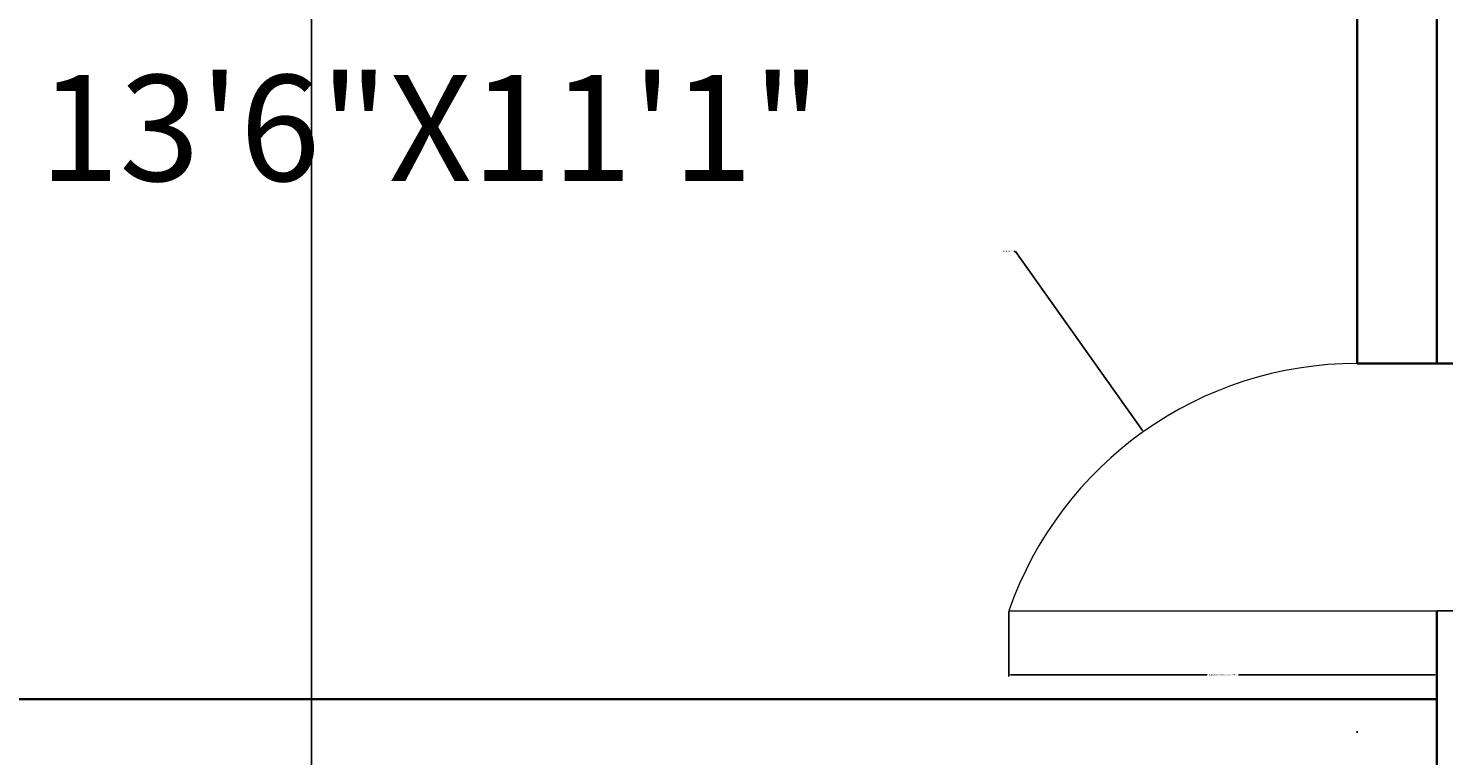
# Model space of a CAD drawing. Units: feet. Extents: x 5816 to 6644, y 25475 to 26788.
# Tile 12 of 23: x 5922 to 6082, y 26514 to 26597. Entities that reach past the tile are written whole.
import ezdxf

# ---------------------------------------------------------------- set-up
doc = ezdxf.new("R2010")
doc.units = ezdxf.units.FT
for name, color, linetype, lineweight in [('A-ANNO-DIMS', 2, 'Continuous', 13), ('A-DOOR', 3, 'Continuous', 18), ('A-WALL', 7, 'Continuous', 35)]:
    doc.layers.add(name, color=color, linetype=linetype, lineweight=lineweight)
doc.styles.get("Standard").update_dxf_attribs({"font": 'arial.ttf'})
doc.dimstyles.get("Standard").update_dxf_attribs({"dimtxt": 0.18, "dimasz": 0.18, "dimexe": 0.18, "dimexo": 0.0625, "dimgap": 0.09, "dimtad": 0, "dimtih": 1, "dimtoh": 1, "dimdec": 4, "dimzin": 0, "dimdsep": 46, "dimtxsty": 'Standard', "dimcen": 0.09, "dimadec": 0, "dimazin": 0, "dimtfac": 1, "dimtdec": 4, "dimtofl": 0, "dimtmove": 0, "dimatfit": 3, "dimfxl": 1, "dimtolj": 1, "dimtzin": 0, "dimarcsym": 0})

# ---------------------------------------------------------------- blocks, each defined once
blk = doc.blocks.new('DOOR-BEDROOM-BALCONY')
blk.add_line((-48.41, 0), (0, 0))
blk.add_arc((-9, -13.73), 41.74, 90, 160.7878)
blk = doc.blocks.new('*D23')
at = {"layer": 'A-ANNO-DIMS', "color": 0, "lineweight": -2, "transparency": 16777216}
for p, q in [((6032.9, 26530.52), (6032.9, 26523.14)), ((6081.31, 26530.52), (6081.31, 26523.14)), ((6033.08, 26523.32), (6055.32, 26523.32)), ((6081.13, 26523.32), (6058.89, 26523.32))]:
    blk.add_line(p, q, dxfattribs=at)
at = {"layer": 'A-ANNO-DIMS', "color": 0, "transparency": 16777216}
for points in [[(6033.08, 26523.35), (6033.08, 26523.29), (6032.9, 26523.32)], [(6081.13, 26523.35), (6081.13, 26523.29), (6081.31, 26523.32)]]:
    blk.add_solid(points, dxfattribs=at)
at = {"layer": 'Defpoints', "color": 0, "transparency": 16777216}
for p in [(6032.9, 26530.58), (6081.31, 26530.58), (6081.31, 26523.32)]:
    blk.add_point(p, dxfattribs=at)
at = {"layer": 'A-ANNO-DIMS', "color": 0, "transparency": 16777216, "insert": (6057.11, 26523.32), "char_height": 0.18, "attachment_point": 5}
blk.add_mtext('\\A1;BALCONY BR DOOR 48 TYP.', dxfattribs=at)
blk = doc.blocks.new('*D24')
at = {"layer": 'A-ANNO-DIMS', "color": 0, "lineweight": -2, "transparency": 16777216}
for p, q in [((6081.37, 26558.58), (6088.75, 26558.58)), ((6088.57, 26558.4), (6088.57, 26544.77)), ((6088.57, 26530.76), (6088.57, 26544.4)), ((6081.37, 26530.58), (6088.75, 26530.58))]:
    blk.add_line(p, q, dxfattribs=at)
at = {"layer": 'A-ANNO-DIMS', "color": 0, "transparency": 16777216}
for points in [[(6088.54, 26558.4), (6088.6, 26558.4), (6088.57, 26558.58)], [(6088.54, 26530.76), (6088.6, 26530.76), (6088.57, 26530.58)]]:
    blk.add_solid(points, dxfattribs=at)
at = {"layer": 'Defpoints', "color": 0, "transparency": 16777216}
for p in [(6081.31, 26558.58), (6088.57, 26558.58), (6081.31, 26530.58)]:
    blk.add_point(p, dxfattribs=at)
at = {"layer": 'A-ANNO-DIMS', "color": 0, "transparency": 16777216, "insert": (6088.57, 26544.58), "char_height": 0.18, "attachment_point": 5}
blk.add_mtext('\\A1;28 TYP.', dxfattribs=at)
blk = doc.blocks.new('*D58')
at = {"layer": 'A-ANNO-DIMS', "color": 0, "lineweight": -2, "transparency": 16777216}
for p, q in [((5953.98, 26168.65), (5953.98, 26787.91)), ((5954.16, 26787.73), (6030.2, 26787.73)), ((6106.8, 26787.73), (6030.76, 26787.73)), ((6106.98, 26168.71), (6106.98, 26787.91))]:
    blk.add_line(p, q, dxfattribs=at)
at = {"layer": 'A-ANNO-DIMS', "color": 0, "transparency": 16777216}
for points in [[(5954.16, 26787.76), (5954.16, 26787.7), (5953.98, 26787.73)], [(6106.8, 26787.76), (6106.8, 26787.7), (6106.98, 26787.73)]]:
    blk.add_solid(points, dxfattribs=at)
at = {"layer": 'Defpoints', "color": 0, "transparency": 16777216}
for p in [(6106.98, 26787.73), (5953.98, 26168.58), (6106.98, 26168.65)]:
    blk.add_point(p, dxfattribs=at)
at = {"layer": 'A-ANNO-DIMS', "color": 0, "transparency": 16777216, "insert": (6030.48, 26787.73), "char_height": 0.18, "attachment_point": 5}
blk.add_mtext('\\A1;153', dxfattribs=at)
blk = doc.blocks.new('*D76')
at = {"layer": 'A-ANNO-DIMS', "color": 0, "lineweight": -2, "transparency": 16777216}
for p, q in [((6033.45, 26571.29), (6033.63, 26571.29)), ((6033.63, 26571.29), (6048.03, 26551.02)), ((6072.22, 26516.85), (6072.4, 26516.85)), ((6072.31, 26516.76), (6072.31, 26516.94))]:
    blk.add_line(p, q, dxfattribs=at)
at = {"layer": 'A-ANNO-DIMS', "color": 0, "transparency": 16777216}
blk.add_solid([(6048.06, 26551.04), (6048.01, 26551), (6048.14, 26550.87)], dxfattribs=at)
at = {"layer": 'Defpoints', "color": 0, "transparency": 16777216}
for p in [(6048.14, 26550.87), (6072.31, 26516.85)]:
    blk.add_point(p, dxfattribs=at)
at = {"layer": 'A-ANNO-DIMS', "color": 0, "transparency": 16777216, "insert": (6032.78, 26571.29), "char_height": 0.18, "attachment_point": 5}
blk.add_mtext('\\A1;4X R41.74', dxfattribs=at)

msp = doc.modelspace()

# ---------------------------------------------------------------- linework, layer by layer
at = {"layer": 'A-WALL'}
for p, q in [((6072.3119, 26558.5846), (6072.3119, 26668.7645)), ((6081.3119, 26558.5846), (6081.3119, 26668.7645)), ((6086.3125, 26558.5846), (6072.3119, 26558.5846)), ((6081.3119, 26520.5846), (6081.3119, 26530.5827)), ((6081.3119, 26530.5827), (6081.3119, 26424.9443)), ((5886.3119, 26520.5846), (6081.3119, 26520.5846))]:
    msp.add_line(p, q, dxfattribs=at)

# ---------------------------------------------------------------- block references
at = {"layer": 'A-DOOR'}
msp.add_blockref('DOOR-BEDROOM-BALCONY', (6081.3119, 26530.5827), dxfattribs=at)

# ---------------------------------------------------------------- texts
at = {"layer": 'A-ANNO-DIMS'}
msp.add_text('13\'6"X11\'1"', height=12, dxfattribs=at).set_placement((5923.1507, 26579.2611))

# ---------------------------------------------------------------- dimensions: what is measured, and where the dimension line sits
dim = msp.add_linear_dim(base=(6106.9781, 26787.7346), p1=(5953.9781, 26168.5846), p2=(6106.9781, 26168.6509), dimstyle='Standard', override={"dimdec": 0, "dimlfac": 1, "dimrnd": 0, "dimzin": 0, "dimdsep": 46, "dimlunit": 2}, dxfattribs=at)
dim.commit()
dim.dimension.update_dxf_attribs({"geometry": '*D58', "text_midpoint": (6030.4781, 26787.7346)})
dim = msp.add_radius_dim(center=(6072.3119, 26516.8487), mpoint=(6048.1387, 26550.8714), text='4X <>', dimstyle='Standard', override={"dimdec": 2, "dimlfac": 1, "dimrnd": 0, "dimzin": 0, "dimdsep": 46, "dimlunit": 2}, dxfattribs=at)
dim.commit()
dim.dimension.update_dxf_attribs({"geometry": '*D76', "text_midpoint": (6032.7783, 26571.2851), "dimtype": 164})
dim = msp.add_linear_dim(base=(6088.5736, 26558.5846), p1=(6081.3119, 26530.5827), p2=(6081.3119, 26558.5846), angle=90, text='<> TYP.', dimstyle='Standard', override={"dimdec": 0, "dimlfac": 1, "dimrnd": 0, "dimzin": 0, "dimdsep": 46, "dimlunit": 2}, dxfattribs=at)
dim.commit()
dim.dimension.update_dxf_attribs({"geometry": '*D24', "text_midpoint": (6088.5736, 26544.5837)})
dim = msp.add_linear_dim(base=(6081.3119, 26523.321), p1=(6032.9004, 26530.5827), p2=(6081.3119, 26530.5827), text='BALCONY BR DOOR <> TYP.', dimstyle='Standard', override={"dimdec": 0, "dimlfac": 1, "dimrnd": 0, "dimzin": 0, "dimdsep": 46, "dimlunit": 2}, dxfattribs=at)
dim.commit()
dim.dimension.update_dxf_attribs({"geometry": '*D23', "text_midpoint": (6057.1061, 26523.321)})

doc.saveas('drawing.dxf')
